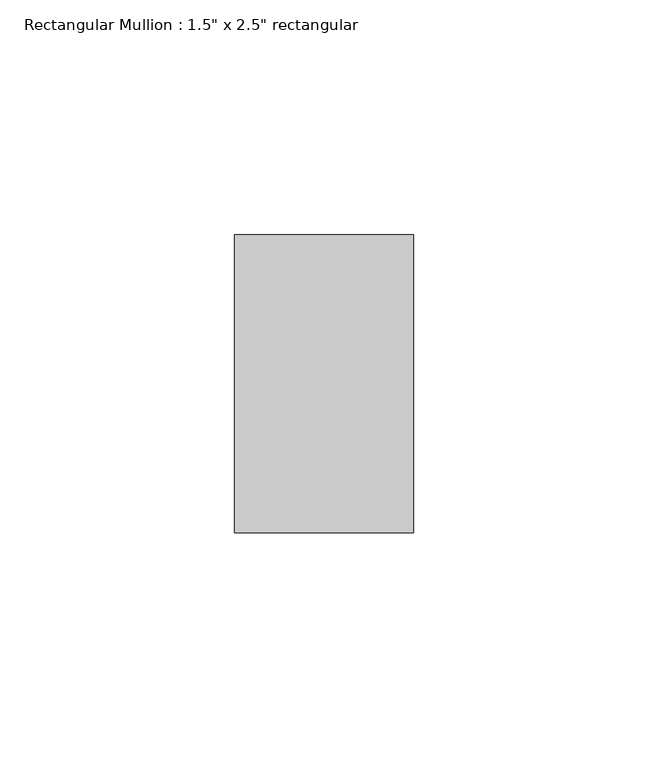
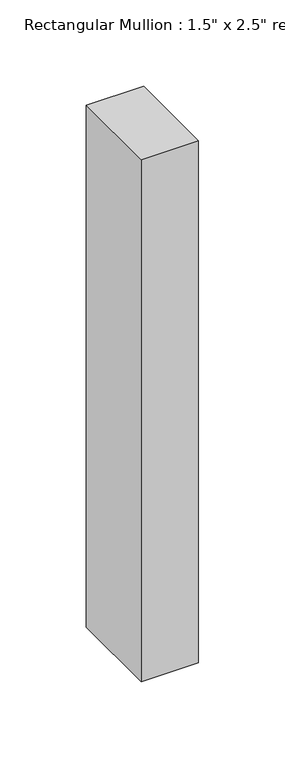
"""IFC4 building model written with IfcOpenShell, lengths in millimetres: member geometry."""

from ifc_helpers import new_model, si_unit, frame, origin, place, context, project, spatial, polyline, outline, extrude, source, transform, mapped, element, save


def member_bec67f52(model_context):
    return source(origin(), model_context, "Body", "SweptSolid", [
        extrude(outline(polyline([(19.05, 31.75), (19.05, -31.75), (-19.05, -31.75), (-19.05, 31.75), (19.05, 31.75)])), frame((0.0, 0.0, -368.3), z_axis=(0.0, 0.0, 1.0), x_axis=(1.0, 0.0, 0.0)), (0.0, 0.0, 1.0), 368.3),
    ])


if __name__ == "__main__":
    model = new_model("IFC4")
    model_context = context("Model", 3, world=origin())
    ifc_project = project(units=[si_unit("LENGTHUNIT", "METRE", prefix="MILLI")], contexts=[model_context])
    site = spatial("IfcSite", under=ifc_project)
    building = spatial("IfcBuilding", under=site)
    placement = place(None, origin())
    member_shape = member_bec67f52(model_context)
    element("IfcMember", 1, ObjectType="Rectangular Mullion : 1.5\" x 2.5\" rectangular", at=placement, inside=building, context=model_context, shape_type="MappedRepresentation", body=[
        mapped(member_shape, transform((0.0, 0.0, 0.0), x_axis=(1.0, 0.0, 0.0), y_axis=(0.0, 1.0, 0.0), z_axis=(0.0, 0.0, 1.0))),
    ])
    save(model, "model.ifc")

# Revit data of these elements
# Type "Rectangular Mullion : 1.5\" x 2.5\" rectangular"
#   built-in parameter 1007304 = 0.208333 (stored number, unit not read)
#   built-in parameter 1007301 = 0.0625 (stored number, unit not read)
#   built-in parameter 1007300 = 0.0625 (stored number, unit not read)
# Element 1 (IfcMember, "Rectangular Mullion : 1.5\" x 2.5\" rectangular")
#   Materials on its faces: "Damp-proofing"
# Materials
#   "Damp-proofing": class "Generic", colour RGB 127 127 127, transparency 0, Description = "Damp-proofing", Cost = 0
